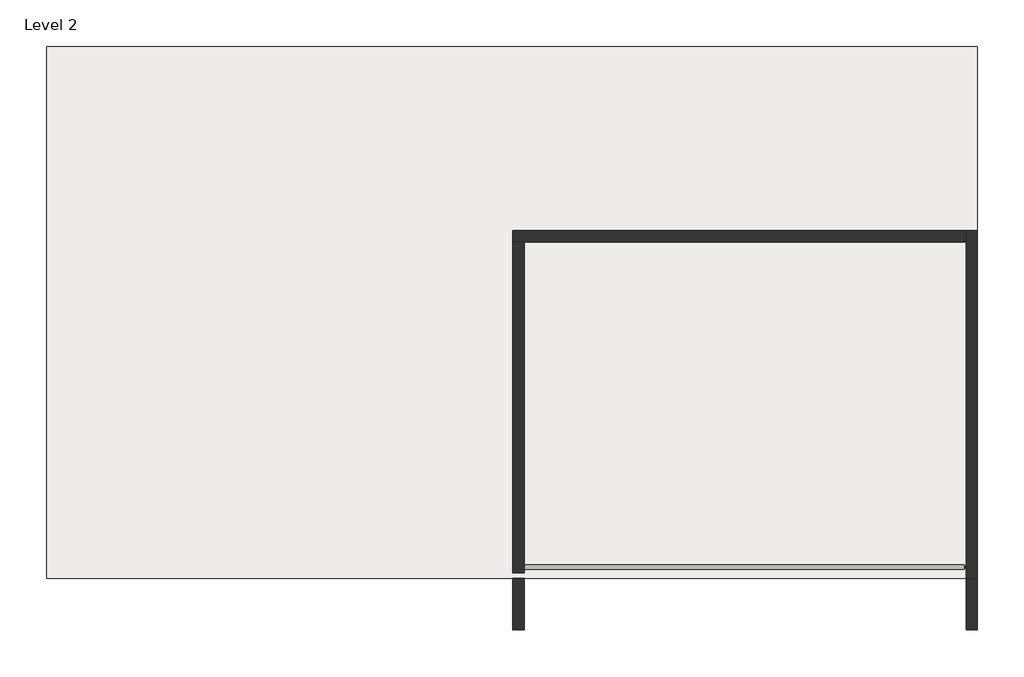
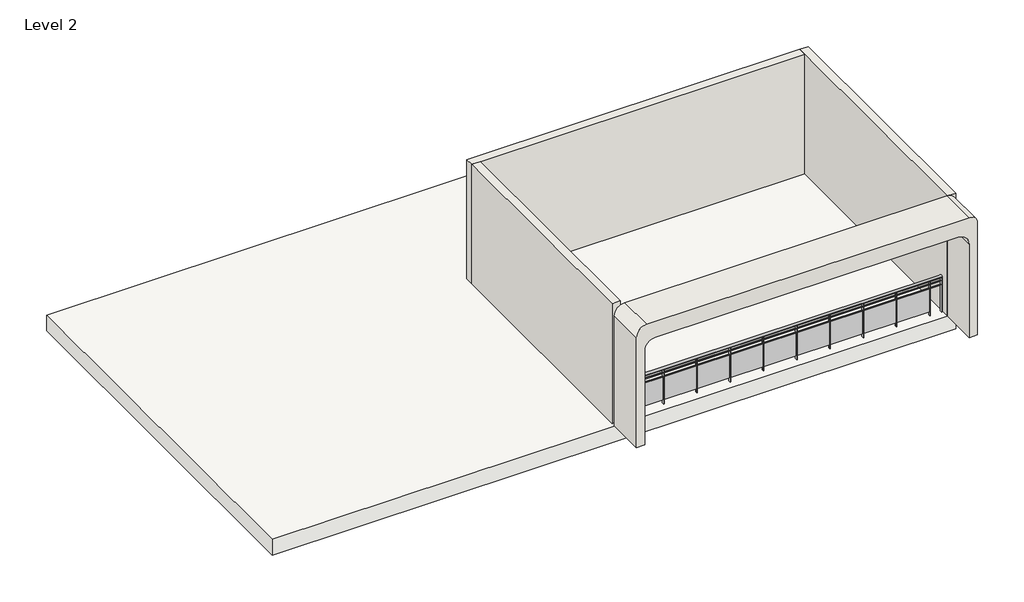
# One storey: 4 walls, 1 railing, 1 slab.
"""IFC4 building model written with IfcOpenShell, lengths in millimetres."""

from ifc_helpers import new_model, si_unit, point, frame, origin, place, context, project, spatial, polyline, ellipse_curve, trimmed, outline, extrude, faceted_brep, transform, mapped, element, save
from ifc_brep_helpers import plane_surface, extruded_surface, advanced_brep
from components import walls_2_walls_2_336146d7

model = new_model("IFC4")

# Units and contexts
model_context = context("Model", 3, world=origin())
ifc_project = project(units=[si_unit("LENGTHUNIT", "METRE", prefix="MILLI")], contexts=[model_context])

# Site, building, storey
site = spatial("IfcSite", under=ifc_project)
building = spatial("IfcBuilding", under=site)
storey = spatial("IfcBuildingStorey", under=building, Name="Level 2", Elevation=6096.0)

# Railing
placement = place(None, origin())
element("IfcRailing", 1, ObjectType="Glass Panel - Bottom Fill", at=placement, inside=storey, context=model_context, shape_type="SolidModel", body=[
    advanced_brep(
    [(3860.4261575, -2899.3603274, 6996.0), (3860.4261575, -2979.3603274, 6996.0), (11632.8261575, -2899.3603274, 6996.0), (11632.8261575, -2979.3603274, 6996.0)],
    [
        (0, 1, ellipse_curve(frame((3860.4261575, -2939.3603274, 6996.0), z_axis=(-1.0, 0.0, 0.0), x_axis=(0.0, -1.0, 0.0)), 40.0, 30.0)),
        (1, 0, ellipse_curve(frame((3860.4261575, -2939.3603274, 6996.0), z_axis=(-1.0, 0.0, 0.0), x_axis=(0.0, -1.0, 0.0)), 40.0, 30.0)),
        (2, 3, ellipse_curve(frame((11632.8261575, -2939.3603274, 6996.0), z_axis=(1.0, 0.0, 0.0), x_axis=(0.0, -1.0, 0.0)), 40.0, 30.0)),
        (3, 2, ellipse_curve(frame((11632.8261575, -2939.3603274, 6996.0), z_axis=(1.0, 0.0, 0.0), x_axis=(0.0, -1.0, 0.0)), 40.0, 30.0)),
        (1, 3),
        (2, 0),
    ],
    [
        plane_surface(frame((3860.4261575, -2939.3603274, 6996.0), z_axis=(-1.0, 0.0, 0.0), x_axis=(0.0, 1.0, 0.0))),
        plane_surface(frame((11632.8261575, -2939.3603274, 6996.0), z_axis=(1.0, 0.0, 0.0), x_axis=(0.0, 1.0, 0.0))),
        extruded_surface(trimmed(ellipse_curve(frame((11632.8261575, -2939.3603274, 6996.0), z_axis=(-1.0, 0.0, 0.0), x_axis=(0.0, -1.0, 0.0)), 40.0, 30.0), [point((11632.8261575, -2979.3603274, 6996.0))], [point((11632.8261575, -2899.3603274, 6996.0))], True, "CARTESIAN"), (-7772.4, 0.0, 0.0), 7772.4),
        extruded_surface(trimmed(ellipse_curve(frame((11632.8261575, -2939.3603274, 6996.0), z_axis=(-1.0, 0.0, 0.0), x_axis=(0.0, -1.0, 0.0)), 40.0, 30.0), [point((11632.8261575, -2899.3603274, 6996.0))], [point((11632.8261575, -2979.3603274, 6996.0))], True, "CARTESIAN"), (-7772.4, 0.0, 0.0), 7772.4),
    ],
    [
        (0, [[1, 2]]),
        (1, [[3, 4]]),
        (2, [[-2, 5, -3, 6]]),
        (3, [[-1, -6, -4, -5]]),
    ],
),
    extrude(outline(polyline([(3860.4261575, -2948.7510925), (3860.4261575, -2928.7510925), (11632.8261575, -2928.7510925), (11632.8261575, -2948.7510925), (3860.4261575, -2948.7510925)])), frame((0.0, 0.0, 6876.0), z_axis=(0.0, 0.0, 1.0), x_axis=(1.0, 0.0, 0.0)), (0.0, 0.0, 1.0), 20.0),
    extrude(outline(polyline([(3860.4261575, -2948.7510925), (3860.4261575, -2928.7510925), (11632.8261575, -2928.7510925), (11632.8261575, -2948.7510925), (3860.4261575, -2948.7510925)])), frame((0.0, 0.0, 6776.0), z_axis=(0.0, 0.0, 1.0), x_axis=(1.0, 0.0, 0.0)), (0.0, 0.0, 1.0), 20.0),
    extrude(outline(polyline([(11340.6261575, -2913.7510925), (11352.6261575, -2913.7510925), (11352.6261575, -2963.7510925), (11340.6261575, -2963.7510925), (11340.6261575, -2913.7510925)])), frame((0.0, 0.0, 6096.0), z_axis=(0.0, 0.0, 1.0), x_axis=(1.0, 0.0, 0.0)), (0.0, 0.0, 1.0), 869.8465326),
    extrude(outline(polyline([(10546.6261575, -2940.4759026), (11346.6261575, -2940.4759026), (11346.6261575, -2945.4759026), (10546.6261575, -2945.4759026), (10546.6261575, -2940.4759026)])), frame((0.0, 0.0, 6196.0), z_axis=(0.0, 0.0, 1.0), x_axis=(1.0, 0.0, 0.0)), (0.0, 0.0, 1.0), 580.0),
    extrude(outline(polyline([(10540.6261575, -2913.7510925), (10552.6261575, -2913.7510925), (10552.6261575, -2963.7510925), (10540.6261575, -2963.7510925), (10540.6261575, -2913.7510925)])), frame((0.0, 0.0, 6096.0), z_axis=(0.0, 0.0, 1.0), x_axis=(1.0, 0.0, 0.0)), (0.0, 0.0, 1.0), 869.8465326),
    extrude(outline(polyline([(9746.6261575, -2940.4759026), (10546.6261575, -2940.4759026), (10546.6261575, -2945.4759026), (9746.6261575, -2945.4759026), (9746.6261575, -2940.4759026)])), frame((0.0, 0.0, 6196.0), z_axis=(0.0, 0.0, 1.0), x_axis=(1.0, 0.0, 0.0)), (0.0, 0.0, 1.0), 580.0),
    extrude(outline(polyline([(9740.6261575, -2913.7510925), (9752.6261575, -2913.7510925), (9752.6261575, -2963.7510925), (9740.6261575, -2963.7510925), (9740.6261575, -2913.7510925)])), frame((0.0, 0.0, 6096.0), z_axis=(0.0, 0.0, 1.0), x_axis=(1.0, 0.0, 0.0)), (0.0, 0.0, 1.0), 869.8465326),
    extrude(outline(polyline([(8946.6261575, -2940.4759026), (9746.6261575, -2940.4759026), (9746.6261575, -2945.4759026), (8946.6261575, -2945.4759026), (8946.6261575, -2940.4759026)])), frame((0.0, 0.0, 6196.0), z_axis=(0.0, 0.0, 1.0), x_axis=(1.0, 0.0, 0.0)), (0.0, 0.0, 1.0), 580.0),
    extrude(outline(polyline([(8940.6261575, -2913.7510925), (8952.6261575, -2913.7510925), (8952.6261575, -2963.7510925), (8940.6261575, -2963.7510925), (8940.6261575, -2913.7510925)])), frame((0.0, 0.0, 6096.0), z_axis=(0.0, 0.0, 1.0), x_axis=(1.0, 0.0, 0.0)), (0.0, 0.0, 1.0), 869.8465326),
    extrude(outline(polyline([(8146.6261575, -2940.4759026), (8946.6261575, -2940.4759026), (8946.6261575, -2945.4759026), (8146.6261575, -2945.4759026), (8146.6261575, -2940.4759026)])), frame((0.0, 0.0, 6196.0), z_axis=(0.0, 0.0, 1.0), x_axis=(1.0, 0.0, 0.0)), (0.0, 0.0, 1.0), 580.0),
    extrude(outline(polyline([(8140.6261575, -2913.7510925), (8152.6261575, -2913.7510925), (8152.6261575, -2963.7510925), (8140.6261575, -2963.7510925), (8140.6261575, -2913.7510925)])), frame((0.0, 0.0, 6096.0), z_axis=(0.0, 0.0, 1.0), x_axis=(1.0, 0.0, 0.0)), (0.0, 0.0, 1.0), 869.8465326),
    extrude(outline(polyline([(7346.6261575, -2940.4759026), (8146.6261575, -2940.4759026), (8146.6261575, -2945.4759026), (7346.6261575, -2945.4759026), (7346.6261575, -2940.4759026)])), frame((0.0, 0.0, 6196.0), z_axis=(0.0, 0.0, 1.0), x_axis=(1.0, 0.0, 0.0)), (0.0, 0.0, 1.0), 580.0),
    extrude(outline(polyline([(7340.6261575, -2913.7510925), (7352.6261575, -2913.7510925), (7352.6261575, -2963.7510925), (7340.6261575, -2963.7510925), (7340.6261575, -2913.7510925)])), frame((0.0, 0.0, 6096.0), z_axis=(0.0, 0.0, 1.0), x_axis=(1.0, 0.0, 0.0)), (0.0, 0.0, 1.0), 869.8465326),
    extrude(outline(polyline([(6546.6261575, -2940.4759026), (7346.6261575, -2940.4759026), (7346.6261575, -2945.4759026), (6546.6261575, -2945.4759026), (6546.6261575, -2940.4759026)])), frame((0.0, 0.0, 6196.0), z_axis=(0.0, 0.0, 1.0), x_axis=(1.0, 0.0, 0.0)), (0.0, 0.0, 1.0), 580.0),
    extrude(outline(polyline([(6540.6261575, -2913.7510925), (6552.6261575, -2913.7510925), (6552.6261575, -2963.7510925), (6540.6261575, -2963.7510925), (6540.6261575, -2913.7510925)])), frame((0.0, 0.0, 6096.0), z_axis=(0.0, 0.0, 1.0), x_axis=(1.0, 0.0, 0.0)), (0.0, 0.0, 1.0), 869.8465326),
    extrude(outline(polyline([(5746.6261575, -2940.4759026), (6546.6261575, -2940.4759026), (6546.6261575, -2945.4759026), (5746.6261575, -2945.4759026), (5746.6261575, -2940.4759026)])), frame((0.0, 0.0, 6196.0), z_axis=(0.0, 0.0, 1.0), x_axis=(1.0, 0.0, 0.0)), (0.0, 0.0, 1.0), 580.0),
    extrude(outline(polyline([(5740.6261575, -2913.7510925), (5752.6261575, -2913.7510925), (5752.6261575, -2963.7510925), (5740.6261575, -2963.7510925), (5740.6261575, -2913.7510925)])), frame((0.0, 0.0, 6096.0), z_axis=(0.0, 0.0, 1.0), x_axis=(1.0, 0.0, 0.0)), (0.0, 0.0, 1.0), 869.8465326),
    extrude(outline(polyline([(4946.6261575, -2940.4759026), (5746.6261575, -2940.4759026), (5746.6261575, -2945.4759026), (4946.6261575, -2945.4759026), (4946.6261575, -2940.4759026)])), frame((0.0, 0.0, 6196.0), z_axis=(0.0, 0.0, 1.0), x_axis=(1.0, 0.0, 0.0)), (0.0, 0.0, 1.0), 580.0),
    extrude(outline(polyline([(4940.6261575, -2913.7510925), (4952.6261575, -2913.7510925), (4952.6261575, -2963.7510925), (4940.6261575, -2963.7510925), (4940.6261575, -2913.7510925)])), frame((0.0, 0.0, 6096.0), z_axis=(0.0, 0.0, 1.0), x_axis=(1.0, 0.0, 0.0)), (0.0, 0.0, 1.0), 869.8465326),
    extrude(outline(polyline([(4146.6261575, -2940.4759026), (4946.6261575, -2940.4759026), (4946.6261575, -2945.4759026), (4146.6261575, -2945.4759026), (4146.6261575, -2940.4759026)])), frame((0.0, 0.0, 6196.0), z_axis=(0.0, 0.0, 1.0), x_axis=(1.0, 0.0, 0.0)), (0.0, 0.0, 1.0), 580.0),
    extrude(outline(polyline([(4140.6261575, -2913.7510925), (4152.6261575, -2913.7510925), (4152.6261575, -2963.7510925), (4140.6261575, -2963.7510925), (4140.6261575, -2913.7510925)])), frame((0.0, 0.0, 6096.0), z_axis=(0.0, 0.0, 1.0), x_axis=(1.0, 0.0, 0.0)), (0.0, 0.0, 1.0), 869.8465326),
    extrude(outline(polyline([(11624.8261575, -2913.7510925), (11636.8261575, -2913.7510925), (11636.8261575, -2963.7510925), (11624.8261575, -2963.7510925), (11624.8261575, -2913.7510925)])), frame((0.0, 0.0, 6096.0), z_axis=(0.0, 0.0, 1.0), x_axis=(1.0, 0.0, 0.0)), (0.0, 0.0, 1.0), 869.8465326),
    extrude(outline(polyline([(3856.4261575, -2913.7510925), (3868.4261575, -2913.7510925), (3868.4261575, -2963.7510925), (3856.4261575, -2963.7510925), (3856.4261575, -2913.7510925)])), frame((0.0, 0.0, 6096.0), z_axis=(0.0, 0.0, 1.0), x_axis=(1.0, 0.0, 0.0)), (0.0, 0.0, 1.0), 869.8465326),
])

# Slab
element("IfcSlab", 2, ObjectType="Generic Floor - 400mm", at=placement, inside=storey, context=model_context, shape_type="SweptSolid", body=[
    extrude(outline(polyline([(11861.7023789, 6257.6489075), (11861.7023789, -3138.7510925), (-4569.1738425, -3138.7510925), (-4569.1738425, 6257.6489075), (11861.7023789, 6257.6489075)])), frame((0.0, 0.0, 5696.0), z_axis=(0.0, 0.0, 1.0), x_axis=(1.0, 0.0, 0.0)), (0.0, 0.0, 1.0), 400.0),
])

# Walls
element("IfcWall", 3, ObjectType="Generic - 9\"", at=placement, inside=storey, context=model_context, shape_type="Brep", body=[
    faceted_brep([(11861.7023789, -3138.7510925, 6096.0), (11861.7023789, 3004.8489075, 6096.0), (11861.7023789, 3004.8489075, 9144.0), (11861.7023789, -3138.7510925, 9144.0), (11661.7023789, -3138.7510925, 6096.0), (11661.7023789, -3138.7510925, 9144.0), (11661.7023789, 2804.8489075, 9144.0), (11661.7023789, 3004.8489075, 9144.0), (11661.7023789, 3004.8489075, 6096.0), (11661.7023789, 2804.8489075, 6096.0)], [[[0, 1, 2, 3]], [[4, 5, 6, 7, 8, 9]], [[1, 0, 4, 9, 8]], [[3, 2, 7, 6, 5]], [[0, 3, 5, 4]], [[2, 1, 8, 7]]]),
])
element("IfcWall", 4, ObjectType="Generic - 9\"", at=placement, inside=storey, context=model_context, shape_type="SweptSolid", body=[
    extrude(outline(polyline([(3660.4261575, -3038.7510925), (3660.4261575, 2804.8489075), (3860.4261575, 2804.8489075), (3860.4261575, -3038.7510925), (3660.4261575, -3038.7510925)])), frame((0.0, 0.0, 6096.0), z_axis=(0.0, 0.0, 1.0), x_axis=(1.0, 0.0, 0.0)), (0.0, 0.0, 1.0), 3048.0),
])
element("IfcWall", 5, ObjectType="Generic - 9\"", at=placement, inside=storey, context=model_context, shape_type="Brep", body=[
    faceted_brep([(3660.4261575, 2804.8489075, 6096.0), (3860.4261575, 2804.8489075, 6096.0), (11661.7023789, 2804.8489075, 6096.0), (11661.7023789, 2804.8489075, 9144.0), (3860.4261575, 2804.8489075, 9144.0), (3660.4261575, 2804.8489075, 9144.0), (3660.4261575, 3004.8489075, 6096.0), (3660.4261575, 3004.8489075, 9144.0), (11661.7023789, 3004.8489075, 9144.0), (11661.7023789, 3004.8489075, 6096.0)], [[[0, 1, 2, 3, 4, 5]], [[6, 7, 8, 9]], [[2, 1, 0, 6, 9]], [[5, 4, 3, 8, 7]], [[3, 2, 9, 8]], [[0, 5, 7, 6]]]),
])
walls_2_walls_2_shape = walls_2_walls_2_336146d7(model_context)
element("IfcWall", 6, ObjectType="Walls 2 : Walls 2", at=placement, inside=storey, context=model_context, shape_type="MappedRepresentation", body=[
    mapped(walls_2_walls_2_shape, transform((0.0, 0.0, 0.0), x_axis=(1.0, 0.0, 0.0), y_axis=(0.0, 1.0, 0.0), z_axis=(0.0, 0.0, 1.0))),
])

save(model, "model.ifc")

# Revit data of these elements
# Type "Glass Panel - Bottom Fill"
#   built-in parameter 1008612 = 0.019685 (stored number, unit not read)
#   built-in parameter 1008611 = 0.019685 (stored number, unit not read)
#   built-in parameter 1008609 = 0.902231 (stored number, unit not read)
#   built-in parameter 1008604 = 0.19685 (stored number, unit not read)
#   built-in parameter 1008603 = 0.164042 (stored number, unit not read)
#   Railing Height = 2' - 11.43307"
#   built-in parameter 1008630 = 2
#   built-in parameter 1008610 = 2
# Type "Generic Floor - 400mm"
#   Function = 0
#   Layers, outside or top first: 1' - 3.74803" no material (function 1)
# Type "Generic - 9\""
#   Layers, outside or top first: 0' - 7.87402" no material (function 1)
# Element 1 (IfcRailing, "Glass Panel - Bottom Fill")
#   Phase Created = New Construction
#   Materials on its faces: "Metal - Stainless Steel,Polished", "Glass"
# Element 2 (IfcSlab, "Generic Floor - 400mm")
#   Height Offset From Level = 0' - 0"
#   Phase Created = New Construction
#   Materials on its faces: "Default Roof"
# Elements 3, 4, 5 (IfcWall, "Generic - 9\"")
#   Top Offset = 0' - 0"
#   Base Offset = 0' - 0"
#   Unconnected Height = 10' - 0"
#   wall height = 10' - 0"
#   Phase Created = New Construction
#   Base Constraint = Level 2
#   Materials on its faces: "Default Wall"
# Element 6 (IfcWall, "Walls 2 : Walls 2")
#   Phase Created = New Construction
#   Materials on its faces: "Default Wall"
# Materials
#   "Metal - Stainless Steel,Polished": class "Metal", colour RGB 189 187 185, transparency 0, Cost = 0
#   "Glass": class "Glass", colour RGB 218 227 224, transparency 0.85, Description = "Soda Lime Glass", Cost = 0
#   "Default Roof": colour RGB 80 80 80, transparency 0
#   "Default Wall": colour RGB 80 80 80, transparency 0
